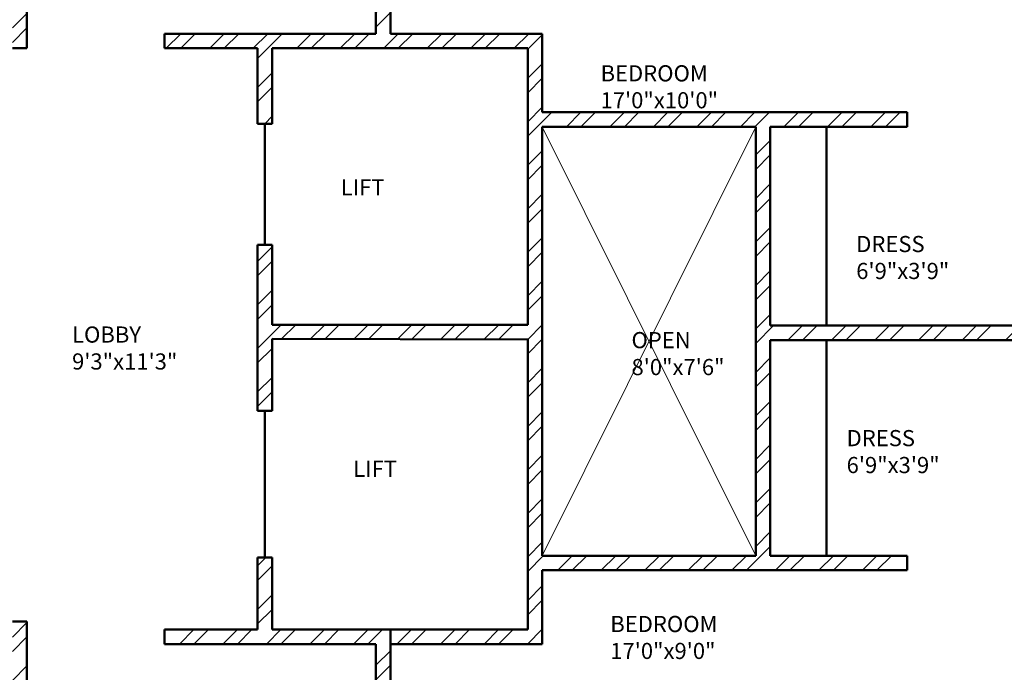
# Model space of a CAD drawing. Units: inches. Extents: x 963 to 2075, y 289 to 2657.
# Tile 57 of 98: x 1511 to 1815, y 1915 to 2117. Entities that reach past the tile are written whole.
import ezdxf

# ---------------------------------------------------------------- set-up
doc = ezdxf.new("R2010")
doc.units = ezdxf.units.IN
for name, color, linetype, lineweight in [('A-ANNO-SYMB', 2, 'Continuous', 18), ('A-AREA-IDEN', 7, 'Continuous', 18), ('A-WALL', 7, 'Continuous', 50), ('A-WALL-PATT', 8, 'Continuous', 13)]:
    doc.layers.add(name, color=color, linetype=linetype, lineweight=lineweight)
doc.styles.get("Standard").update_dxf_attribs({"font": 'arial.ttf'})

msp = doc.modelspace()

# ---------------------------------------------------------------- hatches: boundary and pattern name
at = {"layer": 'A-WALL-PATT'}
h = msp.add_hatch(dxfattribs=at)
h.set_pattern_fill('ANSI32', color=256)
h.paths.add_polyline_path([(1296.92, 2558.32), (1203.92, 2558.32), (1203.92, 2493.82), (1191.53, 2493.82), (1191.53, 2489.32), (1211.06, 2489.32), (1211.06, 2492.02), (1211.06, 2493.82), (1208.42, 2493.82), (1208.42, 2553.82), (1292.42, 2553.82), (1292.42, 2538.86), (1296.92, 2538.86)])
h.paths.add_polyline_path([(1442.42, 2558.32), (1349.42, 2558.32), (1349.42, 2538.94), (1353.92, 2538.94), (1353.92, 2553.82), (1437.92, 2553.82), (1437.92, 2493.82), (1434.54, 2493.82), (1434.54, 2489.32), (1448.31, 2489.32), (1448.31, 2491.57), (1448.31, 2493.82), (1442.42, 2493.82)])
h.paths.add_polyline_path([(1415.55, 2491.57), (1415.55, 2493.82), (1340.94, 2493.82), (1340.94, 2489.32), (1371.92, 2489.32), (1371.92, 2378.32), (1367.6, 2378.32), (1367.6, 2373.82), (1371.92, 2373.82), (1371.92, 2355.19), (1376.42, 2355.19), (1376.42, 2489.32), (1415.55, 2489.32)])
h.paths.add_polyline_path([(1304.94, 2491.57), (1304.94, 2493.82), (1296.92, 2493.82), (1296.92, 2514.86), (1292.42, 2514.86), (1292.42, 2493.82), (1232.81, 2493.82), (1232.81, 2489.32), (1256.42, 2489.32), (1256.42, 2327.32), (1253.71, 2327.32), (1253.71, 2322.82), (1328.42, 2322.82), (1328.42, 2331.15), (1323.92, 2331.15), (1323.92, 2327.32), (1260.92, 2327.32), (1260.92, 2373.82), (1323.92, 2373.82), (1323.92, 2357.81), (1328.42, 2357.81), (1328.42, 2373.82), (1346.01, 2373.82), (1346.01, 2376.07), (1346.01, 2378.32), (1260.92, 2378.32), (1260.92, 2489.32), (1304.94, 2489.32)])
h.paths.add_polyline_path([(1226.65, 2327.32), (1124.42, 2327.32), (1124.42, 2347.45), (1119.92, 2347.45), (1119.92, 2322.82), (1163.42, 2322.82), (1163.42, 2305.43), (1165.67, 2305.43), (1167.92, 2305.43), (1167.92, 2322.82), (1226.65, 2322.82), (1226.65, 2325.07)])
h.paths.add_polyline_path([(1095.92, 2489.32), (1124.42, 2489.32), (1131.53, 2489.32), (1131.53, 2491.57), (1131.53, 2493.82), (1119.92, 2493.82), (1091.42, 2493.82), (1091.42, 2417.32), (1095.92, 2417.32), (1119.92, 2417.32), (1119.92, 2407.45), (1124.42, 2407.45), (1124.42, 2421.82), (1095.92, 2421.82)])
h.paths.add_polyline_path([(1512.92, 2558.32), (1508.42, 2558.32), (1508.42, 2493.82), (1503.4, 2493.82), (1503.4, 2489.32), (1508.42, 2489.32), (1508.42, 2327.32), (1376.42, 2327.32), (1376.42, 2330.27), (1371.92, 2330.27), (1371.92, 2298.74), (1376.42, 2298.74), (1376.42, 2322.82), (1508.42, 2322.82), (1508.42, 2165.32), (1504.26, 2165.32), (1504.26, 2160.82), (1508.42, 2160.82), (1508.42, 2108.32), (1512.92, 2108.32), (1512.92, 2160.82), (1516.18, 2160.82), (1516.18, 2163.07), (1516.18, 2165.32), (1512.92, 2165.32), (1512.92, 2322.82), (1644.92, 2322.82), (1644.92, 2298.74), (1649.42, 2298.74), (1649.42, 2322.82), (1649.42, 2330.94), (1647.17, 2330.94), (1644.92, 2330.94), (1644.92, 2327.32), (1512.92, 2327.32), (1512.92, 2489.32), (1516.76, 2489.32), (1516.76, 2491.57), (1516.76, 2493.82), (1512.92, 2493.82)])
h.paths.add_polyline_path([(1671.92, 2558.32), (1578.92, 2558.32), (1578.92, 2493.82), (1573.53, 2493.82), (1573.53, 2489.32), (1586.54, 2489.32), (1586.54, 2491.57), (1586.54, 2493.82), (1583.42, 2493.82), (1583.42, 2553.82), (1667.42, 2553.82), (1667.42, 2541.11), (1671.92, 2541.11)])
h.paths.add_polyline_path([(1681.26, 2493.82), (1671.92, 2493.82), (1671.92, 2517.11), (1667.42, 2517.11), (1667.42, 2493.82), (1610.22, 2493.82), (1610.22, 2489.32), (1644.92, 2489.32), (1644.92, 2357.87), (1649.42, 2357.87), (1649.42, 2373.82), (1652.2, 2373.82), (1652.2, 2375.83), (1652.2, 2378.32), (1649.42, 2378.32), (1649.42, 2489.32), (1681.26, 2489.32), (1681.26, 2491.57)])
h.paths.add_polyline_path([(1821.92, 2558.32), (1728.92, 2558.32), (1728.92, 2541), (1733.42, 2541), (1733.42, 2553.82), (1817.42, 2553.82), (1817.42, 2493.82), (1813.51, 2493.82), (1813.51, 2489.32), (1830.08, 2489.32), (1830.08, 2491.57), (1830.08, 2493.82), (1821.92, 2493.82)])
h.paths.add_polyline_path([(1794.24, 2493.82), (1717.26, 2493.82), (1717.26, 2489.32), (1760.42, 2489.32), (1760.42, 2378.32), (1674.4, 2378.32), (1674.4, 2373.82), (1692.92, 2373.82), (1692.92, 2356.95), (1697.42, 2356.95), (1697.42, 2373.82), (1760.42, 2373.82), (1760.42, 2327.32), (1697.42, 2327.32), (1697.42, 2333.34), (1692.92, 2333.34), (1692.92, 2322.82), (1768.04, 2322.82), (1768.04, 2325.07), (1768.04, 2327.32), (1764.92, 2327.32), (1764.92, 2489.32), (1794.24, 2489.32)])
h.paths.add_polyline_path([(1733.42, 2517), (1728.92, 2517), (1728.92, 2493.82), (1733.42, 2493.82)], flags=17)
h.paths.add_polyline_path([(1929.92, 2493.82), (1890.08, 2493.82), (1890.08, 2489.32), (1896.92, 2489.32), (1925.42, 2489.32), (1925.42, 2421.82), (1896.92, 2421.82), (1896.92, 2408.32), (1901.42, 2408.32), (1901.42, 2417.32), (1925.42, 2417.32), (1929.92, 2417.32)])
h.paths.add_polyline_path([(1901.42, 2348.32), (1896.92, 2348.32), (1896.92, 2327.32), (1800.42, 2327.32), (1800.42, 2322.82), (1853.42, 2322.82), (1853.42, 2309.45), (1857.92, 2309.45), (1857.92, 2322.82), (1901.42, 2322.82)])
h.paths.add_polyline_path([(1857.92, 2249.45), (1853.42, 2249.45), (1853.42, 2214.82), (1686.31, 2214.82), (1686.31, 2210.32), (1853.42, 2210.32), (1853.42, 2202.13), (1857.92, 2202.13), (1857.92, 2210.32)])
h.paths.add_polyline_path([(1857.92, 2142.13), (1853.42, 2142.13), (1853.42, 2115.42), (1841.42, 2115.42), (1841.42, 2088.53), (1841.42, 2046.95), (1845.92, 2046.95), (1845.92, 2110.92), (1905.92, 2110.92), (1905.92, 2092.52), (1910.42, 2092.52), (1910.42, 2115.42), (1857.92, 2115.42)])
h.paths.add_polyline_path([(1532.44, 1482.34), (1573.46, 1482.34), (1573.46, 1501), (1532.44, 1501)], flags=9)
h.paths.add_polyline_path([(1438.66, 1486.3), (1479.68, 1486.3), (1479.68, 1504.96), (1438.66, 1504.96)], flags=9)
h.paths.add_polyline_path([(1411.22, 1365.31), (1659.14, 1365.31), (1659.14, 1402.4), (1411.22, 1402.4)], flags=9)
h.paths.add_polyline_path([(1185.67, 2296.3), (1248.16, 2296.3), (1248.16, 2314.95), (1185.67, 2314.95)], flags=9)
h.paths.add_polyline_path([(1177.31, 2187.35), (1216.15, 2187.35), (1216.15, 2206.01), (1177.31, 2206.01)], flags=9)
h.paths.add_polyline_path([(1295.1, 1602.08), (1328.26, 1602.08), (1328.26, 1620.74), (1295.1, 1620.74)], flags=9)
h.paths.add_polyline_path([(1525.13, 2005.99), (1558.39, 2005.99), (1558.39, 2024.65), (1525.13, 2024.65)], flags=9)
h.paths.add_polyline_path([(1459.61, 1977.13), (1472.19, 1977.13), (1472.19, 1987.43), (1459.61, 1987.43)], flags=9)
h.paths.add_polyline_path([(1467.81, 2053.68), (1480.02, 2053.68), (1480.02, 2063.98), (1467.81, 2063.98)], flags=9)
h.paths.add_polyline_path([(1555.18, 2119.02), (1584.56, 2119.02), (1584.56, 2137.68), (1555.18, 2137.68)], flags=25)
h.paths.add_polyline_path([(1405.39, 2115.29), (1444.48, 2115.29), (1444.48, 2133.95), (1405.39, 2133.95)], flags=25)
h.paths.add_polyline_path([(1698.48, 2004.26), (1727.69, 2004.26), (1727.69, 2022.92), (1698.48, 2022.92)], flags=9)
h.paths.add_polyline_path([(1612.16, 1972.86), (1629.02, 1972.86), (1629.02, 1983.16), (1612.16, 1983.16)], flags=9)
h.paths.add_polyline_path([(1608.29, 2060.04), (1625.15, 2060.04), (1625.15, 2070.34), (1608.29, 2070.34)], flags=9)
h.paths.add_polyline_path([(1527.95, 1684.4), (1566.79, 1684.4), (1566.79, 1703.06), (1527.95, 1703.06)], flags=9)
h.paths.add_polyline_path([(1422.79, 1683.59), (1461.63, 1683.59), (1461.63, 1702.25), (1422.79, 1702.25)], flags=9)
h.paths.add_polyline_path([(1531.26, 1732.46), (1574.01, 1732.46), (1574.01, 1751.12), (1531.26, 1751.12)], flags=9)
h.paths.add_polyline_path([(1402.87, 1732.85), (1439.8, 1732.85), (1439.8, 1751.5), (1402.87, 1751.5)], flags=9)
h.paths.add_polyline_path([(1243.12, 1923.13), (1281.96, 1923.13), (1281.96, 1941.79), (1243.12, 1941.79)], flags=9)
h.paths.add_polyline_path([(1181.75, 1792.27), (1244.24, 1792.27), (1244.24, 1810.93), (1181.75, 1810.93)], flags=9)
h.paths.add_polyline_path([(1265.82, 1670.3), (1316.07, 1670.3), (1316.07, 1688.96), (1265.82, 1688.96)], flags=9)
h.paths.add_polyline_path([(1140.26, 1676.05), (1179.1, 1676.05), (1179.1, 1694.71), (1140.26, 1694.71)], flags=9)
h.paths.add_polyline_path([(1107.49, 1490.89), (1143.37, 1490.89), (1143.37, 1509.55), (1107.49, 1509.55)], flags=9)
h.paths.add_polyline_path([(1217.58, 1483.9), (1246.74, 1483.9), (1246.74, 1502.56), (1217.58, 1502.56)], flags=9)
h.paths.add_polyline_path([(1389.21, 1486.92), (1418.37, 1486.92), (1418.37, 1505.58), (1389.21, 1505.58)], flags=9)
h.paths.add_polyline_path([(1672.21, 1602.08), (1705.37, 1602.08), (1705.37, 1620.74), (1672.21, 1620.74)], flags=9)
h.paths.add_polyline_path([(1752.08, 1522.64), (1781.24, 1522.64), (1781.24, 1541.3), (1752.08, 1541.3)], flags=9)
h.paths.add_polyline_path([(1848.27, 1491.26), (1884.16, 1491.26), (1884.16, 1509.92), (1848.27, 1509.92)], flags=9)
h.paths.add_polyline_path([(1822.47, 1685.62), (1861.31, 1685.62), (1861.31, 1704.28), (1822.47, 1704.28)], flags=9)
h.paths.add_polyline_path([(1713.19, 1672.23), (1763.44, 1672.23), (1763.44, 1690.89), (1713.19, 1690.89)], flags=9)
h.paths.add_polyline_path([(1736.62, 1790.58), (1799.11, 1790.58), (1799.11, 1809.24), (1736.62, 1809.24)], flags=9)
h.paths.add_polyline_path([(1691.49, 1916.36), (1730.33, 1916.36), (1730.33, 1935.01), (1691.49, 1935.01)], flags=9)
h.paths.add_polyline_path([(1764.87, 1973.92), (1794.31, 1973.92), (1794.31, 1992.58), (1764.87, 1992.58)], flags=9)
h.paths.add_polyline_path([(1767.85, 2034.02), (1797.29, 2034.02), (1797.29, 2052.67), (1767.85, 2052.67)], flags=9)
h.paths.add_polyline_path([(1851.59, 2060.33), (1880.75, 2060.33), (1880.75, 2078.99), (1851.59, 2078.99)], flags=25)
h.paths.add_polyline_path([(1688.49, 2086.87), (1727.33, 2086.87), (1727.33, 2105.53), (1688.49, 2105.53)], flags=9)
h.paths.add_polyline_path([(1537.74, 2293.58), (1580.49, 2293.58), (1580.49, 2312.24), (1537.74, 2312.24)], flags=25)
h.paths.add_polyline_path([(1425.59, 2296.11), (1468.34, 2296.11), (1468.34, 2314.77), (1425.59, 2314.77)], flags=25)
h.paths.add_polyline_path([(1278.52, 2004.18), (1307.72, 2004.18), (1307.72, 2022.84), (1278.52, 2022.84)], flags=9)
h.paths.add_polyline_path([(1193.28, 1973.63), (1222.72, 1973.63), (1222.72, 1992.29), (1193.28, 1992.29)], flags=9)
h.paths.add_polyline_path([(1192.41, 2040.58), (1221.84, 2040.58), (1221.84, 2059.23), (1192.41, 2059.23)], flags=9)
h.paths.add_polyline_path([(1130.6, 1951.39), (1159.76, 1951.39), (1159.76, 1970.05), (1130.6, 1970.05)], flags=9)
h.paths.add_polyline_path([(1132.83, 2052.49), (1161.98, 2052.49), (1161.98, 2071.15), (1132.83, 2071.15)], flags=9)
h.paths.add_polyline_path([(1265.13, 2334.62), (1315.38, 2334.62), (1315.38, 2353.28), (1265.13, 2353.28)], flags=25)
h.paths.add_polyline_path([(1136.74, 2330.79), (1175.58, 2330.79), (1175.58, 2349.44), (1136.74, 2349.44)], flags=9)
h.paths.add_polyline_path([(1287.42, 2417.2), (1320.58, 2417.2), (1320.58, 2435.86), (1287.42, 2435.86)], flags=25)
h.paths.add_polyline_path([(1430.99, 2329.16), (1469.83, 2329.16), (1469.83, 2347.82), (1430.99, 2347.82)], flags=25)
h.paths.add_polyline_path([(1525.42, 2329.21), (1564.26, 2329.21), (1564.26, 2347.87), (1525.42, 2347.87)], flags=25)
h.paths.add_polyline_path([(1684.52, 2382.8), (1717.68, 2382.8), (1717.68, 2401.46), (1684.52, 2401.46)], flags=25)
h.paths.add_polyline_path([(1704.81, 2340.29), (1755.05, 2340.29), (1755.05, 2358.95), (1704.81, 2358.95)], flags=25)
h.paths.add_polyline_path([(1694.11, 2287.76), (1756.6, 2287.76), (1756.6, 2306.41), (1694.11, 2306.41)], flags=9)
h.paths.add_polyline_path([(1815.78, 2329.86), (1854.62, 2329.86), (1854.62, 2348.52), (1815.78, 2348.52)], flags=9)
h.paths.add_polyline_path([(1842.87, 2514.26), (1878.76, 2514.26), (1878.76, 2532.91), (1842.87, 2532.91)], flags=9)
h.paths.add_polyline_path([(1769.51, 2531.45), (1798.67, 2531.45), (1798.67, 2550.1), (1769.51, 2550.1)], flags=25)
h.paths.add_polyline_path([(1594.77, 2518.47), (1623.93, 2518.47), (1623.93, 2537.13), (1594.77, 2537.13)], flags=25)
h.paths.add_polyline_path([(1520.72, 2516.18), (1556.61, 2516.18), (1556.61, 2534.84), (1520.72, 2534.84)], flags=25)
h.paths.add_polyline_path([(1464.46, 2516.69), (1500.34, 2516.69), (1500.34, 2535.35), (1464.46, 2535.35)], flags=25)
h.paths.add_polyline_path([(1365.7, 2528.97), (1394.85, 2528.97), (1394.85, 2547.63), (1365.7, 2547.63)], flags=25)
h.paths.add_polyline_path([(1222.84, 2516.23), (1252, 2516.23), (1252, 2534.89), (1222.84, 2534.89)], flags=25)
h.paths.add_polyline_path([(1104.55, 2509.6), (1140.43, 2509.6), (1140.43, 2528.26), (1104.55, 2528.26)], flags=9)
h = msp.add_hatch(dxfattribs=at)
h.set_pattern_fill('ANSI32', color=256)
h.paths.add_polyline_path([(1335.97, 2212.57), (1335.97, 2214.82), (1167.92, 2214.82), (1167.92, 2245.43), (1163.42, 2245.43), (1163.42, 2210.32), (1163.42, 2194.81), (1167.92, 2194.81), (1167.92, 2210.32), (1335.97, 2210.32)])
h.paths.add_polyline_path([(1532.44, 1482.34), (1573.46, 1482.34), (1573.46, 1501), (1532.44, 1501)], flags=9)
h.paths.add_polyline_path([(1438.66, 1486.3), (1479.68, 1486.3), (1479.68, 1504.96), (1438.66, 1504.96)], flags=9)
h.paths.add_polyline_path([(1411.22, 1365.31), (1659.14, 1365.31), (1659.14, 1402.4), (1411.22, 1402.4)], flags=9)
h.paths.add_polyline_path([(1185.67, 2296.3), (1248.16, 2296.3), (1248.16, 2314.95), (1185.67, 2314.95)], flags=9)
h.paths.add_polyline_path([(1177.31, 2187.35), (1216.15, 2187.35), (1216.15, 2206.01), (1177.31, 2206.01)], flags=9)
h.paths.add_polyline_path([(1295.1, 1602.08), (1328.26, 1602.08), (1328.26, 1620.74), (1295.1, 1620.74)], flags=9)
h.paths.add_polyline_path([(1525.13, 2005.99), (1558.39, 2005.99), (1558.39, 2024.65), (1525.13, 2024.65)], flags=9)
h.paths.add_polyline_path([(1459.61, 1977.13), (1472.19, 1977.13), (1472.19, 1987.43), (1459.61, 1987.43)], flags=9)
h.paths.add_polyline_path([(1467.81, 2053.68), (1480.02, 2053.68), (1480.02, 2063.98), (1467.81, 2063.98)], flags=9)
h.paths.add_polyline_path([(1555.18, 2119.02), (1584.56, 2119.02), (1584.56, 2137.68), (1555.18, 2137.68)], flags=9)
h.paths.add_polyline_path([(1405.39, 2115.29), (1444.48, 2115.29), (1444.48, 2133.95), (1405.39, 2133.95)], flags=9)
h.paths.add_polyline_path([(1698.48, 2004.26), (1727.69, 2004.26), (1727.69, 2022.92), (1698.48, 2022.92)], flags=9)
h.paths.add_polyline_path([(1612.16, 1972.86), (1629.02, 1972.86), (1629.02, 1983.16), (1612.16, 1983.16)], flags=9)
h.paths.add_polyline_path([(1608.29, 2060.04), (1625.15, 2060.04), (1625.15, 2070.34), (1608.29, 2070.34)], flags=9)
h.paths.add_polyline_path([(1527.95, 1684.4), (1566.79, 1684.4), (1566.79, 1703.06), (1527.95, 1703.06)], flags=9)
h.paths.add_polyline_path([(1422.79, 1683.59), (1461.63, 1683.59), (1461.63, 1702.25), (1422.79, 1702.25)], flags=9)
h.paths.add_polyline_path([(1531.26, 1732.46), (1574.01, 1732.46), (1574.01, 1751.12), (1531.26, 1751.12)], flags=9)
h.paths.add_polyline_path([(1402.87, 1732.85), (1439.8, 1732.85), (1439.8, 1751.5), (1402.87, 1751.5)], flags=9)
h.paths.add_polyline_path([(1243.12, 1923.13), (1281.96, 1923.13), (1281.96, 1941.79), (1243.12, 1941.79)], flags=9)
h.paths.add_polyline_path([(1181.75, 1792.27), (1244.24, 1792.27), (1244.24, 1810.93), (1181.75, 1810.93)], flags=9)
h.paths.add_polyline_path([(1265.82, 1670.3), (1316.07, 1670.3), (1316.07, 1688.96), (1265.82, 1688.96)], flags=9)
h.paths.add_polyline_path([(1140.26, 1676.05), (1179.1, 1676.05), (1179.1, 1694.71), (1140.26, 1694.71)], flags=9)
h.paths.add_polyline_path([(1107.49, 1490.89), (1143.37, 1490.89), (1143.37, 1509.55), (1107.49, 1509.55)], flags=9)
h.paths.add_polyline_path([(1217.58, 1483.9), (1246.74, 1483.9), (1246.74, 1502.56), (1217.58, 1502.56)], flags=9)
h.paths.add_polyline_path([(1389.21, 1486.92), (1418.37, 1486.92), (1418.37, 1505.58), (1389.21, 1505.58)], flags=9)
h.paths.add_polyline_path([(1672.21, 1602.08), (1705.37, 1602.08), (1705.37, 1620.74), (1672.21, 1620.74)], flags=9)
h.paths.add_polyline_path([(1752.08, 1522.64), (1781.24, 1522.64), (1781.24, 1541.3), (1752.08, 1541.3)], flags=9)
h.paths.add_polyline_path([(1848.27, 1491.26), (1884.16, 1491.26), (1884.16, 1509.92), (1848.27, 1509.92)], flags=9)
h.paths.add_polyline_path([(1822.47, 1685.62), (1861.31, 1685.62), (1861.31, 1704.28), (1822.47, 1704.28)], flags=9)
h.paths.add_polyline_path([(1713.19, 1672.23), (1763.44, 1672.23), (1763.44, 1690.89), (1713.19, 1690.89)], flags=9)
h.paths.add_polyline_path([(1736.62, 1790.58), (1799.11, 1790.58), (1799.11, 1809.24), (1736.62, 1809.24)], flags=9)
h.paths.add_polyline_path([(1691.49, 1916.36), (1730.33, 1916.36), (1730.33, 1935.01), (1691.49, 1935.01)], flags=9)
h.paths.add_polyline_path([(1764.87, 1973.92), (1794.31, 1973.92), (1794.31, 1992.58), (1764.87, 1992.58)], flags=9)
h.paths.add_polyline_path([(1767.85, 2034.02), (1797.29, 2034.02), (1797.29, 2052.67), (1767.85, 2052.67)], flags=9)
h.paths.add_polyline_path([(1851.59, 2060.33), (1880.75, 2060.33), (1880.75, 2078.99), (1851.59, 2078.99)], flags=9)
h.paths.add_polyline_path([(1688.49, 2086.87), (1727.33, 2086.87), (1727.33, 2105.53), (1688.49, 2105.53)], flags=9)
h.paths.add_polyline_path([(1537.74, 2293.58), (1580.49, 2293.58), (1580.49, 2312.24), (1537.74, 2312.24)], flags=9)
h.paths.add_polyline_path([(1425.59, 2296.11), (1468.34, 2296.11), (1468.34, 2314.77), (1425.59, 2314.77)], flags=9)
h.paths.add_polyline_path([(1278.52, 2004.18), (1307.72, 2004.18), (1307.72, 2022.84), (1278.52, 2022.84)], flags=9)
h.paths.add_polyline_path([(1193.28, 1973.63), (1222.72, 1973.63), (1222.72, 1992.29), (1193.28, 1992.29)], flags=9)
h.paths.add_polyline_path([(1192.41, 2040.58), (1221.84, 2040.58), (1221.84, 2059.23), (1192.41, 2059.23)], flags=9)
h.paths.add_polyline_path([(1130.6, 1951.39), (1159.76, 1951.39), (1159.76, 1970.05), (1130.6, 1970.05)], flags=9)
h.paths.add_polyline_path([(1132.83, 2052.49), (1161.98, 2052.49), (1161.98, 2071.15), (1132.83, 2071.15)], flags=9)
h.paths.add_polyline_path([(1265.13, 2334.62), (1315.38, 2334.62), (1315.38, 2353.28), (1265.13, 2353.28)], flags=9)
h.paths.add_polyline_path([(1136.74, 2330.79), (1175.58, 2330.79), (1175.58, 2349.44), (1136.74, 2349.44)], flags=9)
h.paths.add_polyline_path([(1287.42, 2417.2), (1320.58, 2417.2), (1320.58, 2435.86), (1287.42, 2435.86)], flags=9)
h.paths.add_polyline_path([(1430.99, 2329.16), (1469.83, 2329.16), (1469.83, 2347.82), (1430.99, 2347.82)], flags=9)
h.paths.add_polyline_path([(1525.42, 2329.21), (1564.26, 2329.21), (1564.26, 2347.87), (1525.42, 2347.87)], flags=9)
h.paths.add_polyline_path([(1684.52, 2382.8), (1717.68, 2382.8), (1717.68, 2401.46), (1684.52, 2401.46)], flags=9)
h.paths.add_polyline_path([(1704.81, 2340.29), (1755.05, 2340.29), (1755.05, 2358.95), (1704.81, 2358.95)], flags=9)
h.paths.add_polyline_path([(1694.11, 2287.76), (1756.6, 2287.76), (1756.6, 2306.41), (1694.11, 2306.41)], flags=9)
h.paths.add_polyline_path([(1815.78, 2329.86), (1854.62, 2329.86), (1854.62, 2348.52), (1815.78, 2348.52)], flags=9)
h.paths.add_polyline_path([(1842.87, 2514.26), (1878.76, 2514.26), (1878.76, 2532.91), (1842.87, 2532.91)], flags=9)
h.paths.add_polyline_path([(1769.51, 2531.45), (1798.67, 2531.45), (1798.67, 2550.1), (1769.51, 2550.1)], flags=9)
h.paths.add_polyline_path([(1594.77, 2518.47), (1623.93, 2518.47), (1623.93, 2537.13), (1594.77, 2537.13)], flags=9)
h.paths.add_polyline_path([(1520.72, 2516.18), (1556.61, 2516.18), (1556.61, 2534.84), (1520.72, 2534.84)], flags=9)
h.paths.add_polyline_path([(1464.46, 2516.69), (1500.34, 2516.69), (1500.34, 2535.35), (1464.46, 2535.35)], flags=9)
h.paths.add_polyline_path([(1365.7, 2528.97), (1394.85, 2528.97), (1394.85, 2547.63), (1365.7, 2547.63)], flags=9)
h.paths.add_polyline_path([(1222.84, 2516.23), (1252, 2516.23), (1252, 2534.89), (1222.84, 2534.89)], flags=9)
h.paths.add_polyline_path([(1104.55, 2509.6), (1140.43, 2509.6), (1140.43, 2528.26), (1104.55, 2528.26)], flags=9)
h = msp.add_hatch(dxfattribs=at)
h.set_pattern_fill('ANSI32', color=256)
h.paths.add_polyline_path([(1473.61, 2163.07), (1473.61, 2165.32), (1376.42, 2165.32), (1376.42, 2227.98), (1371.92, 2227.98), (1371.92, 2214.82), (1368.41, 2214.82), (1368.41, 2210.32), (1371.92, 2210.32), (1371.92, 2160.82), (1395.92, 2160.82), (1395.92, 2090.32), (1217.34, 2090.32), (1217.34, 2085.82), (1395.92, 2085.82), (1458.92, 2085.82), (1458.92, 2108.32), (1454.42, 2108.32), (1454.42, 2090.32), (1400.42, 2090.32), (1400.42, 2160.82), (1473.61, 2160.82)])
h.paths.add_polyline_path([(1649.42, 2210.32), (1653.23, 2210.32), (1653.23, 2214.82), (1649.42, 2214.82), (1649.42, 2227.98), (1644.92, 2227.98), (1644.92, 2165.32), (1550.1, 2165.32), (1550.1, 2160.82), (1620.92, 2160.82), (1620.92, 2112.82), (1555.45, 2112.82), (1555.45, 2108.32), (1584.33, 2108.32), (1584.33, 2084.92), (1588.83, 2084.92), (1588.83, 2108.32), (1625.42, 2108.32), (1667.95, 2108.32), (1667.95, 2022.67), (1588.83, 2022.67), (1588.83, 2047.41), (1584.33, 2047.41), (1584.33, 1996), (1588.83, 1996), (1588.83, 2018.32), (1667.95, 2018.17), (1667.95, 1928.32), (1625.42, 1928.32), (1625.42, 1923.82), (1672.45, 1923.82), (1672.45, 1928.32), (1672.45, 1946.66), (1785.45, 1946.66), (1785.45, 1951.16), (1743.03, 1951.16), (1743.03, 2017.92), (1841.42, 2017.92), (1841.42, 2014.77), (1845.92, 2014.77), (1845.92, 2017.92), (1905.92, 2017.92), (1905.92, 1987.51), (1910.42, 1987.51), (1910.42, 2022.42), (1910.42, 2068.52), (1905.92, 2068.52), (1905.92, 2022.42), (1845.92, 2022.42), (1845.92, 2025.85), (1843.67, 2025.85), (1841.42, 2025.85), (1841.42, 2022.42), (1743.03, 2022.42), (1743.03, 2084.03), (1768.45, 2084.03), (1785.45, 2084.03), (1785.45, 2088.53), (1672.45, 2088.53), (1672.45, 2112.82), (1667.95, 2112.82), (1625.42, 2112.82), (1625.42, 2160.82), (1649.42, 2160.82)])
h.paths.add_polyline_path([(1672.45, 2084.03), (1738.53, 2084.03), (1738.53, 1951.16), (1672.45, 1951.16)], flags=16)
h.paths.add_polyline_path([(1672.45, 2084.03), (1738.53, 2084.03), (1705.49, 2017.6)], flags=0)
h.paths.add_polyline_path([(1262.77, 2085.82), (1258.27, 2085.82), (1258.27, 2023.28), (1184.42, 2023.28), (1184.42, 2018.78), (1258.27, 2018.78), (1258.27, 1950.82), (1262.77, 1950.82)])
h.paths.add_polyline_path([(1312.27, 2085.82), (1307.77, 2085.82), (1307.77, 1950.82), (1312.27, 1950.82)])
h.paths.add_polyline_path([(1458.92, 1950.82), (1395.92, 1950.82), (1216.57, 1950.82), (1216.57, 1946.32), (1346.42, 1946.32), (1395.92, 1946.32), (1395.92, 1875.82), (1371.92, 1875.82), (1371.92, 1826.32), (1368.93, 1826.32), (1368.93, 1821.82), (1371.92, 1821.82), (1371.92, 1813.62), (1376.42, 1813.62), (1376.42, 1871.32), (1474.5, 1871.32), (1474.5, 1873.57), (1474.5, 1875.82), (1400.42, 1875.82), (1400.42, 1946.32), (1454.42, 1946.32), (1454.42, 1928.32), (1458.92, 1928.32)])
h.paths.add_polyline_path([(1184.42, 2120.78), (1167.92, 2120.78), (1167.92, 2134.81), (1165.67, 2134.81), (1163.42, 2134.81), (1163.42, 2120.78), (1119.92, 2120.78), (1119.92, 2098.1), (1124.42, 2098.1), (1124.42, 2116.28), (1167.92, 2116.28), (1179.92, 2116.28), (1179.92, 2045.92), (1184.42, 2045.92), (1184.42, 2090.32), (1184.42, 2116.28)])
h.paths.add_polyline_path([(1124.42, 2018.78), (1179.92, 2018.78), (1179.92, 2016.29), (1184.42, 2016.29), (1184.42, 2023.28), (1184.42, 2026.59), (1182.17, 2026.59), (1179.92, 2026.59), (1179.92, 2023.28), (1124.42, 2023.28), (1124.42, 2074.1), (1119.92, 2074.1), (1119.92, 2018.78), (1119.92, 1979.63), (1124.42, 1979.63)])
h.paths.add_polyline_path([(1184.42, 1925.78), (1184.42, 1946.32), (1184.42, 1996.07), (1182.17, 1996.07), (1179.92, 1996.07), (1179.92, 1925.78), (1124.42, 1925.78), (1124.42, 1955.63), (1119.92, 1955.5), (1119.92, 1921.28), (1158.92, 1921.28), (1158.92, 1909.98), (1163.42, 1909.98), (1163.42, 1921.28), (1184.42, 1921.28)])
h.paths.add_polyline_path([(1341.45, 1826.32), (1163.42, 1826.32), (1163.42, 1849.98), (1158.92, 1849.98), (1158.92, 1821.82), (1158.92, 1804.03), (1163.42, 1804.03), (1163.42, 1821.82), (1341.45, 1821.82)])
h.paths.add_polyline_path([(1222.98, 1713.82), (1163.42, 1713.82), (1163.42, 1744.03), (1161.17, 1744.03), (1158.92, 1744.03), (1158.92, 1713.82), (1119.92, 1713.82), (1119.92, 1694.65), (1124.42, 1694.65), (1124.42, 1709.32), (1158.92, 1709.32), (1222.98, 1709.32)])
h.paths.add_polyline_path([(1328.42, 1713.82), (1252.04, 1713.82), (1252.04, 1711.57), (1252.04, 1709.32), (1256.42, 1709.32), (1256.42, 1547.32), (1232.94, 1547.32), (1232.94, 1545.07), (1232.94, 1542.82), (1292.42, 1542.82), (1292.42, 1527.63), (1296.92, 1527.63), (1296.92, 1542.82), (1299.46, 1542.82), (1299.46, 1547.32), (1260.92, 1547.32), (1260.92, 1658.32), (1343.66, 1658.32), (1343.66, 1660.57), (1343.66, 1662.82), (1328.42, 1662.82), (1328.42, 1676.59), (1327.4, 1676.59), (1323.92, 1676.59), (1323.92, 1662.82), (1260.92, 1662.82), (1260.92, 1709.32), (1323.92, 1709.32), (1323.92, 1699.85), (1328.42, 1699.85)])
h.paths.add_polyline_path([(1649.42, 1875.82), (1625.42, 1875.82), (1625.42, 1928.32), (1620.92, 1928.32), (1588.83, 1928.32), (1588.83, 1950.59), (1584.33, 1950.59), (1584.33, 1928.32), (1555.45, 1928.32), (1555.45, 1923.82), (1620.92, 1923.82), (1620.92, 1875.82), (1548.95, 1875.82), (1548.95, 1873.57), (1548.95, 1871.32), (1644.92, 1871.32), (1644.92, 1813.62), (1649.42, 1813.62), (1649.42, 1821.82), (1652.04, 1821.82), (1652.04, 1824.07), (1652.04, 1826.32), (1649.42, 1826.32)])
h.paths.add_polyline_path([(1512.92, 1871.32), (1516.48, 1871.32), (1516.48, 1875.82), (1512.92, 1875.82), (1512.92, 1923.82), (1512.92, 1928.32), (1512.92, 1930.83), (1508.42, 1930.83), (1508.42, 1875.82), (1504.41, 1875.82), (1504.41, 1871.32), (1508.42, 1871.32), (1508.42, 1713.82), (1376.42, 1713.82), (1376.42, 1743.32), (1371.92, 1743.32), (1371.92, 1709.32), (1371.92, 1706.01), (1376.42, 1706.01), (1376.42, 1709.32), (1508.42, 1709.32), (1508.42, 1547.32), (1501.87, 1547.32), (1501.87, 1542.82), (1508.42, 1542.82), (1508.42, 1482.82), (1508.42, 1436.32), (1512.92, 1436.32), (1512.92, 1542.82), (1519.32, 1542.82), (1519.32, 1545.07), (1519.32, 1547.32), (1512.92, 1547.32), (1512.92, 1709.32), (1644.92, 1709.32), (1644.92, 1707.55), (1649.42, 1707.55), (1649.42, 1709.32), (1649.42, 1743.32), (1644.92, 1743.32), (1644.92, 1713.82), (1512.92, 1713.82)])
h.paths.add_polyline_path([(1129.88, 1545.07), (1129.88, 1547.32), (1124.42, 1547.32), (1095.92, 1547.32), (1095.92, 1614.82), (1124.42, 1614.82), (1124.42, 1619.32), (1095.92, 1619.32), (1091.42, 1619.32), (1091.42, 1542.82), (1095.92, 1542.82), (1119.92, 1542.82), (1129.88, 1542.82)])
h.paths.add_polyline_path([(1208.42, 1542.82), (1211.74, 1542.82), (1211.74, 1547.32), (1198.85, 1547.32), (1198.85, 1542.82), (1203.92, 1542.82), (1203.92, 1478.32), (1208.42, 1478.32), (1296.92, 1478.32), (1296.92, 1503.63), (1292.42, 1503.63), (1292.42, 1482.82), (1208.42, 1482.82)])
h.paths.add_polyline_path([(1430.42, 1542.82), (1435.7, 1542.82), (1435.7, 1545.07), (1435.7, 1547.32), (1422.66, 1547.32), (1422.66, 1545.07), (1422.66, 1542.82), (1425.92, 1542.82), (1425.92, 1482.86), (1341.92, 1482.86), (1341.92, 1502.73), (1337.42, 1502.73), (1337.42, 1478.36), (1425.92, 1478.36), (1425.92, 1440.82), (1425.92, 1436.32), (1430.42, 1436.32)])
h.paths.add_polyline_path([(1698.48, 2004.26), (1727.69, 2004.26), (1727.69, 2022.92), (1698.48, 2022.92)], flags=8)

# ---------------------------------------------------------------- linework, layer by layer
at = {"layer": 'A-ANNO-SYMB'}
for p, q in [((1738.53, 2084.03), (1672.45, 1951.16)), ((1738.53, 1951.16), (1672.45, 2084.03))]:
    msp.add_line(p, q, dxfattribs=at)
at = {"layer": 'A-WALL'}
for p, q in [((1512.92, 2108.32), (1512.92, 2160.82)), ((1620.92, 2112.82), (1620.92, 2160.82)), ((1625.42, 2112.82), (1625.42, 2160.82)), ((1555.45, 2112.82), (1620.92, 2112.82)), ((1555.45, 2112.82), (1555.45, 2108.32)), ((1625.42, 2112.82), (1667.95, 2112.82)), ((1667.95, 2112.82), (1672.45, 2112.82)), ((1672.45, 2112.82), (1672.45, 2088.53)), ((1512.92, 2108.32), (1508.42, 2108.32)), ((1555.45, 2108.32), (1584.33, 2108.32)), ((1584.33, 2084.92), (1584.33, 2108.32)), ((1588.83, 2108.32), (1588.83, 2084.92)), ((1588.83, 2108.32), (1625.42, 2108.32)), ((1667.95, 2108.32), (1622.7, 2108.32)), ((1667.95, 2022.67), (1667.95, 2108.32)), ((1785.45, 2088.53), (1672.45, 2088.53)), ((1785.45, 2088.53), (1785.45, 2084.03)), ((1584.33, 2084.92), (1588.83, 2084.92)), ((1586.58, 2084.92), (1586.58, 2047.41)), ((1672.45, 2084.03), (1738.53, 2084.03)), ((1672.45, 2084.03), (1738.53, 2084.03)), ((1672.45, 2084.03), (1672.45, 1951.16)), ((1738.53, 2084.03), (1738.53, 1951.16)), ((1743.03, 2084.03), (1768.45, 2084.03)), ((1743.03, 2084.03), (1785.45, 2084.03)), ((1743.03, 2022.42), (1743.03, 2084.03)), ((1760.39, 2084.03), (1760.39, 2022.42)), ((1584.33, 2047.41), (1588.83, 2047.41)), ((1584.33, 1996), (1584.33, 2047.41)), ((1588.83, 2047.41), (1588.83, 2022.67)), ((1588.83, 2022.67), (1667.95, 2022.67)), ((1743.03, 2022.42), (1841.42, 2022.42)), ((1667.95, 2018.17), (1588.83, 2018.32)), ((1588.83, 2018.32), (1588.83, 1996)), ((1667.95, 1928.32), (1667.95, 2018.17)), ((1743.03, 1951.16), (1743.03, 2017.92)), ((1841.42, 2017.92), (1743.03, 2017.92)), ((1760.39, 2017.92), (1760.39, 1951.16)), ((1584.33, 1996), (1588.83, 1996)), ((1586.58, 1996), (1586.58, 1950.59)), ((1672.45, 1951.16), (1738.53, 1951.16)), ((1743.03, 1951.16), (1785.45, 1951.16)), ((1768.45, 1951.16), (1772.95, 1951.16)), ((1785.45, 1951.16), (1785.45, 1946.66)), ((1584.33, 1928.32), (1584.33, 1950.59)), ((1584.33, 1950.59), (1588.83, 1950.59)), ((1588.83, 1950.59), (1588.83, 1928.32)), ((1672.45, 1946.66), (1672.45, 1928.32)), ((1785.45, 1946.66), (1672.45, 1946.66)), ((1508.42, 1930.83), (1512.92, 1930.83)), ((1512.92, 1928.32), (1512.92, 1930.83)), ((1512.92, 1923.82), (1512.92, 1928.32)), ((1555.45, 1928.32), (1584.33, 1928.32)), ((1555.45, 1928.32), (1555.45, 1923.82)), ((1588.83, 1928.32), (1620.92, 1928.32)), ((1620.92, 1928.32), (1625.42, 1928.32)), ((1625.42, 1928.32), (1625.42, 1875.82)), ((1625.42, 1928.32), (1667.95, 1928.32)), ((1672.45, 1928.32), (1672.45, 1923.82)), ((1512.92, 1875.82), (1512.92, 1923.82)), ((1620.92, 1923.82), (1555.45, 1923.82)), ((1620.92, 1875.82), (1620.92, 1923.82)), ((1672.45, 1923.82), (1625.42, 1923.82))]:
    msp.add_line(p, q, dxfattribs=at)

# ---------------------------------------------------------------- texts
at = {"layer": 'A-AREA-IDEN', "char_height": 5, "attachment_point": 1}
for s, width, insert in [('BEDROOM\\P17\'0"x10\'0"', 164.9632, (1690.5, 2103.05)), ('LIFT', 132.9836, (1610.05, 2067.77)), ('DRESS\\P6\'9"x3\'9"', 166.9409, (1769.64, 2050.19)), ('LOBBY\\P9\'3"x11\'3"', 221.8114, (1526.89, 2022.16)), ('OPEN\\P8\'0"x7\'6"', 71.355, (1700.07, 2020.43)), ('DRESS\\P6\'9"x3\'9"', 125.8731, (1766.66, 1990.09)), ('LIFT', 94.499, (1613.92, 1980.59)), ('BEDROOM\\P17\'0"x9\'0"', 161.4859, (1693.5, 1932.53))]:
    msp.add_mtext_dynamic_manual_height_columns(s, width=width, gutter_width=12.5, heights=[0], dxfattribs=dict(at, insert=insert))

doc.saveas('drawing.dxf')
